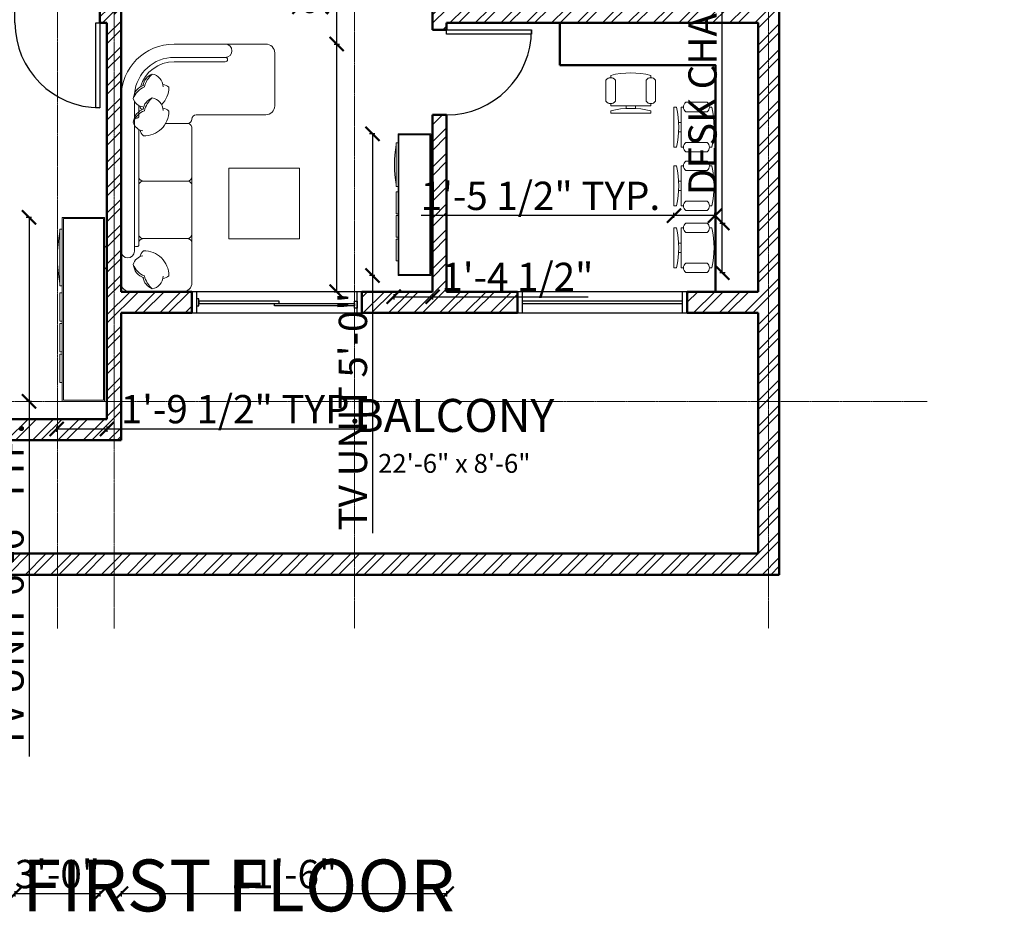
# Model space of a CAD drawing. Units: inches. Extents: x 261 to 2725, y 291 to 1454.
# Tile 23 of 35: x 1407 to 1824, y 296 to 675. Entities that reach past the tile are written whole.
import ezdxf

# ---------------------------------------------------------------- set-up
doc = ezdxf.new("R2010")
doc.units = ezdxf.units.IN
doc.linetypes.add('CENTER', pattern=[2, 1.25, -0.25, 0.25, -0.25])
for name, color, linetype, lineweight in [('A-ANNO-DIMS', 136, 'Continuous', 18), ('A-ANNO-TEXT', 7, 'Continuous', 25), ('A-AREA-IDEN', 18, 'Continuous', 18), ('A-DOOR', 160, 'Continuous', 25), ('A-FLOR-FIXT', 145, 'Continuous', 18), ('A-FURN', 30, 'Continuous', 18), ('A-GLAZ', 150, 'Continuous', 25), ('A-GRID', 251, 'CENTER', 13), ('A-WALL', 222, 'Continuous', 50), ('A-WALL-PATT', 243, 'Continuous', 13)]:
    doc.layers.add(name, color=color, linetype=linetype, lineweight=lineweight)
doc.styles.get("Standard").update_dxf_attribs({"font": 'arial.ttf'})
doc.dimstyles.new('ISO-25', dxfattribs={"dimtxt": 12, "dimasz": 6, "dimexe": 1.25, "dimexo": 0.625, "dimtad": 1, "dimdec": 0, "dimlunit": 3, "dimtxsty": 'Standard', "dimblk": 'ARCHTICK', "dimcen": 2.5, "dimadec": 0, "dimazin": 0, "dimtfac": 1, "dimtdec": 0, "dimtmove": 0, "dimatfit": 3, "dimfxl": 1, "dimfxlon": 1, "dimarcsym": 0})

# ---------------------------------------------------------------- blocks, each defined once
blk = doc.blocks.new('*U6')
for p, q in [((-36, 0), (-36, 6)), ((0, 0), (0, 6))]:
    blk.add_line(p, q)
blk.add_lwpolyline([(0, 0), (0, -36), (-1.75, -36), (-1.75, 0)], close=True)
blk.add_arc((0, 0), 36, 180, 270)
blk = doc.blocks.new('*U13')
for p, q in [((-36, 0), (-36, 6)), ((0, 0), (0, 6))]:
    blk.add_line(p, q)
blk.add_lwpolyline([(0, 0), (0, -36), (-1.75, -36), (-1.75, 0)], close=True)
blk.add_arc((0, 0), 36, 180, 270)
blk = doc.blocks.new('A$C714C64AF')
for p, q in [((3108, 2017, -5499), (1005, 2017, -5499)), ((908, 1917, -5499), (908, 1317, -5499)), ((1365, 1867, -5499), (2793, 1867, -5499)), ((3508, 1417, -5499), (3508, 839, -5499)), ((3558, 1417, -5499), (3558, 839, -5499)), ((3708, 1417, -5499), (3708, 839, -5499)), ((1008, 1217, -5499), (1458, 1217, -5499)), ((1558, 1217, -5499), (1458, 1217, -5499)), ((1558, 1217, -5499), (2760, 1217, -5499)), ((2209, 1217, -5499), (2109, 1217, -5499)), ((2908, 1167, -5499), (2908, 381, -5499)), ((3708, 839, -5499), (3708, 381, -5499)), ((3008, 281, -5499), (3608, 281, -5499))]:
    blk.add_line(p, q)
at = {"elevation": -5499}
for points in [[(940, 1667, -0.14773), (1086, 1753, -0.213343), (1215, 1879)], [(1058, 1544, 0.165541), (1089, 1478, 0.425989), (1370, 1765, 0.121523), (1303, 1804)], [(1066, 1760, -0.306663), (1215, 1879, -0.30633), (1312, 1770)], [(1456, 1817), (1438, 1817, -0.414214), (1418, 1837), (1418, 1847, -0.414214), (1438, 1867)], [(1458, 1817, -0.414214), (1508, 1767)], [(1558, 1817, 0.414214), (1508, 1767), (1508, 1267, 0.432452)], [(1558, 1817, 0.414214), (1508, 1767)], [(2670, 1867), (1884, 1867, 0.414214)], [(2109, 1817, -0.414214), (2159, 1767)], [(2209, 1817, 0.414214), (2159, 1767), (2159, 1267, 0.432452)], [(2209, 1817, 0.414214), (2159, 1767)], [(2982, 1544, -0.165541), (2951, 1478, -0.425989), (2670, 1765, -0.121523), (2737, 1804)], [(2974, 1760, 0.306663), (2825, 1879, 0.30633), (2727, 1770)], [(3068, 1867), (2753, 1867, 0.415492)], [(3100, 1667, 0.14773), (2954, 1753, 0.213343), (2825, 1879)], [(3013, 1867), (2891, 1867, 0.414214), (2871, 1847), (2871, 1837, 0.414214), (2891, 1817), (2963, 1817, 0.414214)], [(2964, 1785, -0.071865), (3006, 1804)], [(3243, 1760, 0.306663), (3094, 1879, 0.30633), (2997, 1770)], [(3369, 1667, 0.14773), (3223, 1753, 0.213343), (3094, 1879)], [(1083, 1541, -0.356772), (940, 1667, -0.249542), (1070, 1771)], [(2957, 1541, 0.356772), (3100, 1667, 0.249542), (2970, 1771)], [(3226, 1541, 0.356772), (3369, 1667, 0.249542), (3239, 1771)], [(3251, 1544, -0.165541), (3220, 1478, -0.200231), (3022, 1559)]]:
    blk.add_lwpolyline(points, format="xyb", dxfattribs=at)
for points in [[(1458, 1817), (2743, 1817)], [(1884, 1867), (2670, 1867)], [(2944, 1817), (3012, 1817)], [(2810, 1515), (2810, 1267)]]:
    blk.add_lwpolyline(points, dxfattribs=at)
blk.add_lwpolyline([(2306, 800), (1506, 800), (1506, 0), (2306, 0)], close=True, dxfattribs=at)
for centre, radius, start, end in [((1008, 1917, -5499), 100, 90, 180), ((1365, 1942, -5499), 75, 90, 270), ((3108, 1417, -5499), 600, 0, 90), ((3108, 1417, -5499), 450, 0, 84.5853), ((3108, 1417, -5499), 400, 0, 72.9371), ((1008, 1317, -5499), 100, 180, 270), ((1458, 1267, -5499), 50, 270, 0), ((1458, 1267, -5499), 50, 270, 0), ((1558, 1267, -5499), 50, 180, 270), ((1558, 1267, -5499), 50, 180, 270), ((2109, 1267, -5499), 50, 270, 0), ((2109, 1267, -5499), 50, 270, 0), ((2209, 1267, -5499), 50, 180, 270), ((2209, 1267, -5499), 50, 180, 270), ((2760, 1267, -5499), 50, 270, 0), ((2760, 1267, -5499), 50, 270, 0), ((2860, 1267, -5499), 50, 180, 270), ((2860, 1267, -5499), 50, 180, 270), ((2858, 1167, -5499), 50, 0, 90), ((3533, 839, -5499), 25, 180, 0), ((3633, 839, -5499), 75, 180, 0), ((3008, 381, -5499), 100, 180, 270), ((3608, 381, -5499), 100, 270, 0)]:
    blk.add_arc(centre, radius, start, end)
blk = doc.blocks.new('Entertainment Center')
for p, q in [((-4, 0), (-5, -1)), ((4, 0), (-4, 0)), ((5, -1), (4, 0)), ((-17, -19), (-17, -1)), ((-17, -1), (61, -1)), ((-16.5, -18.5), (-16.5, -1.5)), ((-16.5, -1.5), (60.5, -1.5)), ((60.5, -1.5), (60.5, -18.5)), ((61, -1), (61, -19)), ((61, -19), (-17, -19)), ((60.5, -18.5), (-16.5, -18.5)), ((-12, -20), (-12, -19)), ((12, -20), (-12, -20)), ((12, -19), (12, -20)), ((15, -20), (15, -19)), ((27, -20), (15, -20)), ((27, -19), (27, -20)), ((28, -20), (28, -19)), ((40, -20), (28, -20)), ((40, -19), (40, -20)), ((41, -20), (41, -19)), ((53, -20), (41, -20)), ((53, -19), (53, -20))]:
    blk.add_line(p, q)
blk.add_arc((0, 40), 61, 259.6111, 280.3889)
blk = doc.blocks.new('Chair - Desk')
for p, q in [((-8.5, 0), (-8.5, -1)), ((-8.5, 0), (8.5, 0)), ((8.5, 0), (8.5, -1)), ((-8.5, -3), (-8.5, -4)), ((-8.5, -3), (8.5, -3)), ((-2, -3), (-2, -1.9355)), ((2, -1.9576), (2, -3)), ((8.5, -3), (8.5, -4)), ((-10.5, -5), (-10.5, -14)), ((-6.5, -14), (-6.5, -5)), ((6.5, -5), (6.5, -14)), ((10.5, -14), (10.5, -5)), ((-8.5, -15), (-8.5, -16)), ((8.5, -15), (8.5, -16))]:
    blk.add_line(p, q)
for centre, radius, start, end in [((-8.5, -6.5), 2.5, 36.8699, 143.1301), ((0, 34.625), 36.625, 256.5803, 283.4197), ((8.5, -6.5), 2.5, 36.8699, 143.1301), ((-8.5, -12.5), 2.5, 216.8699, 323.1301), ((0, 19.625), 36.625, 256.5803, 283.4197), ((8.5, -12.5), 2.5, 216.8699, 323.1301)]:
    blk.add_arc(centre, radius, start, end)
blk = doc.blocks.new('WIN-72')
for p, q in [((955.45, 950.47), (946.45, 950.47)), ((950.45, 950.47), (950.45, 882.47)), ((951.45, 882.47), (951.45, 950.47)), ((946.45, 882.47), (955.45, 882.47))]:
    blk.add_line(p, q)
blk.add_lwpolyline([(955.45, 880.47), (955.45, 952.47), (946.45, 952.47), (946.45, 880.47)], close=True)
blk = doc.blocks.new('DOOR-SLIDING-72')
for p, q in [((1632.08, 973.47), (1632.08, 964.47)), ((1700.08, 964.47), (1700.08, 973.47))]:
    blk.add_line(p, q)
for points in [[(1702.08, 964.47), (1702.08, 973.47), (1630.08, 973.47), (1630.08, 964.47)], [(1632.08, 967.47), (1633.08, 967.47), (1633.08, 970.47), (1632.08, 970.47)], [(1633.08, 968.47), (1667.08, 968.47), (1667.08, 969.47), (1633.08, 969.47)], [(1699.08, 967.47), (1665.08, 967.47), (1665.08, 968.47), (1699.08, 968.47)], [(1700.08, 966.47), (1699.08, 966.47), (1699.08, 969.47), (1700.08, 969.47)]]:
    blk.add_lwpolyline(points, close=True)
blk = doc.blocks.new('_ArchTick')
at = {"color": 0, "linetype": 'ByBlock', "const_width": 0.15}
blk.add_lwpolyline([(-0.5, -0.5), (0.5, 0.5)], dxfattribs=at)
blk = doc.blocks.new('*D43')
at = {"layer": 'A-ANNO-DIMS', "color": 0, "lineweight": -2, "ltscale": 0.07, "transparency": 16777216}
for p, q in [((1412.05, 590.97), (1409.8, 590.97)), ((1411.05, 590.97), (1411.05, 512.97)), ((1412.05, 512.97), (1409.8, 512.97)), ((1411.05, 512.97), (1411.05, 362.42))]:
    blk.add_line(p, q, dxfattribs=at)
at = {"layer": 'Defpoints', "color": 0, "ltscale": 0.07, "transparency": 16777216}
for p in [(1422.75, 590.97), (1411.05, 512.97), (1422.75, 512.97)]:
    blk.add_point(p, dxfattribs=at)
at = {"layer": 'A-ANNO-DIMS', "color": 0, "lineweight": -2, "ltscale": 0.07, "transparency": 16777216, "xscale": 6, "yscale": 6, "zscale": 6}
for p, rotation in [((1411.05, 590.97), 90), ((1411.05, 512.97), 270)]:
    blk.add_blockref('_ArchTick', p, dxfattribs=dict(at, rotation=rotation))
at = {"layer": 'A-ANNO-DIMS', "color": 0, "ltscale": 0.07, "transparency": 16777216, "insert": (1404.29, 434.7), "char_height": 12, "attachment_point": 5, "rotation": 90}
blk.add_mtext('TV UNIT 6\'-6" TYP.', dxfattribs=at)
blk = doc.blocks.new('*D44')
at = {"layer": 'A-ANNO-DIMS', "color": 0, "lineweight": -2, "ltscale": 0.07, "transparency": 16777216}
for p, q in [((1422.75, 502.27), (1422.75, 500.02)), ((1422.75, 501.27), (1444.08, 501.27)), ((1444.08, 502.27), (1444.08, 500.02)), ((1444.08, 501.27), (1551.31, 501.27))]:
    blk.add_line(p, q, dxfattribs=at)
at = {"layer": 'Defpoints', "color": 0, "ltscale": 0.07, "transparency": 16777216}
for p in [(1422.75, 512.97), (1444.08, 512.97), (1444.08, 501.27)]:
    blk.add_point(p, dxfattribs=at)
at = {"layer": 'A-ANNO-DIMS', "color": 0, "lineweight": -2, "ltscale": 0.07, "transparency": 16777216, "xscale": 6, "yscale": 6, "zscale": 6, "rotation": 180}
blk.add_blockref('_ArchTick', (1422.75, 501.27), dxfattribs=at)
at = {"layer": 'A-ANNO-DIMS', "color": 0, "lineweight": -2, "ltscale": 0.07, "transparency": 16777216, "xscale": 6, "yscale": 6, "zscale": 6}
blk.add_blockref('_ArchTick', (1444.08, 501.27), dxfattribs=at)
at = {"layer": 'A-ANNO-DIMS', "color": 0, "ltscale": 0.07, "transparency": 16777216, "insert": (1500.69, 508.1), "char_height": 12, "attachment_point": 5}
blk.add_mtext('1\'-9 1/2" TYP.', dxfattribs=at)
blk = doc.blocks.new('*D45')
at = {"layer": 'A-ANNO-DIMS', "color": 0, "lineweight": -2, "ltscale": 0.07, "transparency": 16777216}
for p, q in [((1557.65, 626.41), (1555.4, 626.41)), ((1556.65, 626.41), (1556.65, 566.36)), ((1557.65, 566.36), (1555.4, 566.36)), ((1556.65, 566.36), (1556.65, 457.06))]:
    blk.add_line(p, q, dxfattribs=at)
at = {"layer": 'Defpoints', "color": 0, "ltscale": 0.07, "transparency": 16777216}
for p in [(1565.66, 626.41), (1556.65, 566.36), (1565.66, 566.36)]:
    blk.add_point(p, dxfattribs=at)
at = {"layer": 'A-ANNO-DIMS', "color": 0, "lineweight": -2, "ltscale": 0.07, "transparency": 16777216, "xscale": 6, "yscale": 6, "zscale": 6}
for p, rotation in [((1556.65, 626.41), 90), ((1556.65, 566.36), 270)]:
    blk.add_blockref('_ArchTick', p, dxfattribs=dict(at, rotation=rotation))
at = {"layer": 'A-ANNO-DIMS', "color": 0, "ltscale": 0.07, "transparency": 16777216, "insert": (1549.9, 508.71), "char_height": 12, "attachment_point": 5, "rotation": 90}
blk.add_mtext('TV UNIT 5\'-0"', dxfattribs=at)
blk = doc.blocks.new('*D46')
at = {"layer": 'A-ANNO-DIMS', "color": 0, "lineweight": -2, "ltscale": 0.07, "transparency": 16777216}
for p, q in [((1565.66, 558.35), (1565.66, 556.1)), ((1565.66, 557.35), (1582.08, 557.35)), ((1582.08, 558.35), (1582.08, 556.1)), ((1582.08, 557.35), (1648.06, 557.35))]:
    blk.add_line(p, q, dxfattribs=at)
at = {"layer": 'Defpoints', "color": 0, "ltscale": 0.07, "transparency": 16777216}
for p in [(1565.66, 566.36), (1582.08, 566.36), (1582.08, 557.35)]:
    blk.add_point(p, dxfattribs=at)
at = {"layer": 'A-ANNO-DIMS', "color": 0, "lineweight": -2, "ltscale": 0.07, "transparency": 16777216, "xscale": 6, "yscale": 6, "zscale": 6, "rotation": 180}
blk.add_blockref('_ArchTick', (1565.66, 557.35), dxfattribs=at)
at = {"layer": 'A-ANNO-DIMS', "color": 0, "lineweight": -2, "ltscale": 0.07, "transparency": 16777216, "xscale": 6, "yscale": 6, "zscale": 6}
blk.add_blockref('_ArchTick', (1582.08, 557.35), dxfattribs=at)
at = {"layer": 'A-ANNO-DIMS', "color": 0, "ltscale": 0.07, "transparency": 16777216, "insert": (1618.07, 564.18), "char_height": 12, "attachment_point": 5}
blk.add_mtext('1\'-4 1/2"', dxfattribs=at)
blk = doc.blocks.new('*D49')
at = {"layer": 'A-ANNO-DIMS', "color": 0, "lineweight": -2, "ltscale": 0.07, "transparency": 16777216}
for p, q in [((1704.93, 588.57), (1704.93, 775.49)), ((1703.93, 588.57), (1706.18, 588.57)), ((1704.93, 567.57), (1704.93, 588.57)), ((1703.93, 567.57), (1706.18, 567.57))]:
    blk.add_line(p, q, dxfattribs=at)
at = {"layer": 'Defpoints', "color": 0, "ltscale": 0.07, "transparency": 16777216}
for p in [(1701.78, 588.57), (1704.93, 588.57), (1701.78, 567.57)]:
    blk.add_point(p, dxfattribs=at)
at = {"layer": 'A-ANNO-DIMS', "color": 0, "lineweight": -2, "ltscale": 0.07, "transparency": 16777216, "xscale": 6, "yscale": 6, "zscale": 6}
for p, rotation in [((1704.93, 588.57), 90), ((1704.93, 567.57), 270)]:
    blk.add_blockref('_ArchTick', p, dxfattribs=dict(at, rotation=rotation))
at = {"layer": 'A-ANNO-DIMS', "color": 0, "ltscale": 0.07, "transparency": 16777216, "insert": (1698.1, 685.03), "char_height": 12, "attachment_point": 5, "rotation": 90}
blk.add_mtext('DESK CHAIR 1\'-9" TYP.', dxfattribs=at)
blk = doc.blocks.new('*D50')
at = {"layer": 'A-ANNO-DIMS', "color": 0, "lineweight": -2, "ltscale": 0.07, "transparency": 16777216}
for p, q in [((1684.45, 590.72), (1684.45, 592.97)), ((1701.78, 590.72), (1701.78, 592.97)), ((1684.45, 591.72), (1577.22, 591.72)), ((1701.78, 591.72), (1684.45, 591.72))]:
    blk.add_line(p, q, dxfattribs=at)
at = {"layer": 'Defpoints', "color": 0, "ltscale": 0.07, "transparency": 16777216}
for p in [(1684.45, 591.72), (1684.45, 588.57), (1701.78, 588.57)]:
    blk.add_point(p, dxfattribs=at)
at = {"layer": 'A-ANNO-DIMS', "color": 0, "lineweight": -2, "ltscale": 0.07, "transparency": 16777216, "xscale": 6, "yscale": 6, "zscale": 6, "rotation": 180}
blk.add_blockref('_ArchTick', (1684.45, 591.72), dxfattribs=at)
at = {"layer": 'A-ANNO-DIMS', "color": 0, "lineweight": -2, "ltscale": 0.07, "transparency": 16777216, "xscale": 6, "yscale": 6, "zscale": 6}
blk.add_blockref('_ArchTick', (1701.78, 591.72), dxfattribs=at)
at = {"layer": 'A-ANNO-DIMS', "color": 0, "ltscale": 0.07, "transparency": 16777216, "insert": (1627.84, 598.55), "char_height": 12, "attachment_point": 5}
blk.add_mtext('1\'-5 1/2" TYP.', dxfattribs=at)
blk = doc.blocks.new('*D55')
at = {"layer": 'A-ANNO-DIMS', "color": 0, "lineweight": -2, "ltscale": 0.07, "transparency": 16777216}
for p, q in [((1541.46, 664.47), (1541.46, 832.37)), ((1540.46, 664.47), (1542.71, 664.47)), ((1541.46, 559.47), (1541.46, 664.47)), ((1540.46, 559.47), (1542.71, 559.47))]:
    blk.add_line(p, q, dxfattribs=at)
at = {"layer": 'Defpoints', "color": 0, "ltscale": 0.07, "transparency": 16777216}
for p in [(1525.71, 664.47), (1541.46, 664.47), (1525.71, 559.47)]:
    blk.add_point(p, dxfattribs=at)
at = {"layer": 'A-ANNO-DIMS', "color": 0, "lineweight": -2, "ltscale": 0.07, "transparency": 16777216, "xscale": 6, "yscale": 6, "zscale": 6}
for p, rotation in [((1541.46, 664.47), 90), ((1541.46, 559.47), 270)]:
    blk.add_blockref('_ArchTick', p, dxfattribs=dict(at, rotation=rotation))
at = {"layer": 'A-ANNO-DIMS', "color": 0, "ltscale": 0.07, "transparency": 16777216, "insert": (1534.63, 751.42), "char_height": 12, "attachment_point": 5, "rotation": 90}
blk.add_mtext('SOFA SET 8\'-9" TYP.', dxfattribs=at)
blk = doc.blocks.new('*D56')
at = {"layer": 'A-ANNO-DIMS', "color": 0, "lineweight": -2, "ltscale": 0.07, "transparency": 16777216}
for p, q in [((1450.08, 679.22), (1450.08, 681.47)), ((1525.71, 679.22), (1525.71, 681.47)), ((1450.08, 680.22), (1341.66, 680.22)), ((1525.71, 680.22), (1450.08, 680.22))]:
    blk.add_line(p, q, dxfattribs=at)
at = {"layer": 'Defpoints', "color": 0, "ltscale": 0.07, "transparency": 16777216}
for p in [(1450.08, 680.22), (1450.08, 664.47), (1525.71, 664.47)]:
    blk.add_point(p, dxfattribs=at)
at = {"layer": 'A-ANNO-DIMS', "color": 0, "lineweight": -2, "ltscale": 0.07, "transparency": 16777216, "xscale": 6, "yscale": 6, "zscale": 6, "rotation": 180}
blk.add_blockref('_ArchTick', (1450.08, 680.22), dxfattribs=at)
at = {"layer": 'A-ANNO-DIMS', "color": 0, "lineweight": -2, "ltscale": 0.07, "transparency": 16777216, "xscale": 6, "yscale": 6, "zscale": 6}
blk.add_blockref('_ArchTick', (1525.71, 680.22), dxfattribs=at)
at = {"layer": 'A-ANNO-DIMS', "color": 0, "ltscale": 0.07, "transparency": 16777216, "insert": (1392.87, 687.05), "char_height": 12, "attachment_point": 5}
blk.add_mtext('6\'-3 1/2" TYP.', dxfattribs=at)
blk = doc.blocks.new('*D82')
at = {"layer": 'A-ANNO-DIMS', "color": 0, "lineweight": -2, "ltscale": 0.07, "transparency": 16777216}
for p, q in [((2600.96, 679.47), (2603.21, 679.47)), ((2601.96, 517.47), (2601.96, 679.47)), ((2600.96, 517.47), (2603.21, 517.47))]:
    blk.add_line(p, q, dxfattribs=at)
at = {"layer": 'Defpoints', "color": 0, "ltscale": 0.07, "transparency": 16777216}
for p in [(946.45, 679.47), (2601.96, 679.47), (946.45, 517.47)]:
    blk.add_point(p, dxfattribs=at)
at = {"layer": 'A-ANNO-DIMS', "color": 0, "lineweight": -2, "ltscale": 0.07, "transparency": 16777216, "xscale": 6, "yscale": 6, "zscale": 6}
for p, rotation in [((2601.96, 679.47), 90), ((2601.96, 517.47), 270)]:
    blk.add_blockref('_ArchTick', p, dxfattribs=dict(at, rotation=rotation))
at = {"layer": 'A-ANNO-DIMS', "color": 0, "ltscale": 0.07, "transparency": 16777216, "insert": (2595.2, 598.47), "char_height": 12, "attachment_point": 5, "rotation": 90}
blk.add_mtext('13\'-6"', dxfattribs=at)
blk = doc.blocks.new('*D89')
at = {"layer": 'A-ANNO-DIMS', "color": 0, "lineweight": -2, "ltscale": 0.07, "transparency": 16777216}
for p, q in [((2600.96, 508.47), (2603.21, 508.47)), ((2601.96, 412.47), (2601.96, 508.47)), ((2600.96, 412.47), (2603.21, 412.47))]:
    blk.add_line(p, q, dxfattribs=at)
at = {"layer": 'Defpoints', "color": 0, "ltscale": 0.07, "transparency": 16777216}
for p in [(955.45, 508.47), (2601.96, 508.47), (994.45, 412.47)]:
    blk.add_point(p, dxfattribs=at)
at = {"layer": 'A-ANNO-DIMS', "color": 0, "lineweight": -2, "ltscale": 0.07, "transparency": 16777216, "xscale": 6, "yscale": 6, "zscale": 6}
for p, rotation in [((2601.96, 508.47), 90), ((2601.96, 412.47), 270)]:
    blk.add_blockref('_ArchTick', p, dxfattribs=dict(at, rotation=rotation))
at = {"layer": 'A-ANNO-DIMS', "color": 0, "ltscale": 0.07, "transparency": 16777216, "insert": (2595.21, 460.47), "char_height": 12, "attachment_point": 5, "rotation": 90}
blk.add_mtext('8\'-0"', dxfattribs=at)
blk = doc.blocks.new('*D111')
at = {"layer": 'A-ANNO-DIMS', "color": 0, "lineweight": -2, "ltscale": 0.07, "transparency": 16777216}
for p, q in [((2600.96, 550.47), (2603.21, 550.47)), ((2601.96, 448.47), (2601.96, 550.47)), ((2600.96, 448.47), (2603.21, 448.47))]:
    blk.add_line(p, q, dxfattribs=at)
at = {"layer": 'Defpoints', "color": 0, "ltscale": 0.07, "transparency": 16777216}
for p in [(1720.08, 550.47), (2601.96, 550.47), (1720.08, 448.47)]:
    blk.add_point(p, dxfattribs=at)
at = {"layer": 'A-ANNO-DIMS', "color": 0, "lineweight": -2, "ltscale": 0.07, "transparency": 16777216, "xscale": 6, "yscale": 6, "zscale": 6}
for p, rotation in [((2601.96, 550.47), 90), ((2601.96, 448.47), 270)]:
    blk.add_blockref('_ArchTick', p, dxfattribs=dict(at, rotation=rotation))
at = {"layer": 'A-ANNO-DIMS', "color": 0, "ltscale": 0.07, "transparency": 16777216, "insert": (2595.21, 499.47), "char_height": 12, "attachment_point": 5, "rotation": 90}
blk.add_mtext('8\'-6"', dxfattribs=at)
blk = doc.blocks.new('*D112')
at = {"layer": 'A-ANNO-DIMS', "color": 0, "lineweight": -2, "ltscale": 0.07, "transparency": 16777216}
for p, q in [((2600.96, 679.47), (2603.21, 679.47)), ((2601.96, 550.47), (2601.96, 679.47)), ((2600.96, 550.47), (2603.21, 550.47))]:
    blk.add_line(p, q, dxfattribs=at)
at = {"layer": 'Defpoints', "color": 0, "ltscale": 0.07, "transparency": 16777216}
for p in [(1720.08, 679.47), (2601.96, 679.47), (1720.08, 550.47)]:
    blk.add_point(p, dxfattribs=at)
at = {"layer": 'A-ANNO-DIMS', "color": 0, "lineweight": -2, "ltscale": 0.07, "transparency": 16777216, "xscale": 6, "yscale": 6, "zscale": 6}
for p, rotation in [((2601.96, 679.47), 90), ((2601.96, 550.47), 270)]:
    blk.add_blockref('_ArchTick', p, dxfattribs=dict(at, rotation=rotation))
at = {"layer": 'A-ANNO-DIMS', "color": 0, "ltscale": 0.07, "transparency": 16777216, "insert": (2595.21, 614.97), "char_height": 12, "attachment_point": 5, "rotation": 90}
blk.add_mtext('10\'-9"', dxfattribs=at)
blk = doc.blocks.new('*D116')
at = {"layer": 'A-ANNO-DIMS', "color": 0, "lineweight": -2, "ltscale": 0.07, "transparency": 16777216}
for p, q in [((1450.08, 305.22), (1450.08, 302.97)), ((1588.08, 305.22), (1588.08, 302.97)), ((1450.08, 304.22), (1588.08, 304.22))]:
    blk.add_line(p, q, dxfattribs=at)
at = {"layer": 'Defpoints', "color": 0, "ltscale": 0.07, "transparency": 16777216}
for p in [(1588.08, 559.47), (1450.08, 550.47), (1588.08, 304.22)]:
    blk.add_point(p, dxfattribs=at)
at = {"layer": 'A-ANNO-DIMS', "color": 0, "lineweight": -2, "ltscale": 0.07, "transparency": 16777216, "xscale": 6, "yscale": 6, "zscale": 6, "rotation": 180}
blk.add_blockref('_ArchTick', (1450.08, 304.22), dxfattribs=at)
at = {"layer": 'A-ANNO-DIMS', "color": 0, "lineweight": -2, "ltscale": 0.07, "transparency": 16777216, "xscale": 6, "yscale": 6, "zscale": 6}
blk.add_blockref('_ArchTick', (1588.08, 304.22), dxfattribs=at)
at = {"layer": 'A-ANNO-DIMS', "color": 0, "ltscale": 0.07, "transparency": 16777216, "insert": (1519.08, 310.97), "char_height": 12, "attachment_point": 5}
blk.add_mtext('11\'-6"', dxfattribs=at)
blk = doc.blocks.new('*D117')
at = {"layer": 'A-ANNO-DIMS', "color": 0, "lineweight": -2, "ltscale": 0.07, "transparency": 16777216}
for p, q in [((1588.08, 1437.76), (1588.08, 1440.01)), ((1702.08, 1437.76), (1702.08, 1440.01)), ((1588.08, 1438.76), (1702.08, 1438.76))]:
    blk.add_line(p, q, dxfattribs=at)
at = {"layer": 'Defpoints', "color": 0, "ltscale": 0.07, "transparency": 16777216}
for p in [(1702.08, 1438.76), (1588.08, 559.47), (1702.08, 559.47)]:
    blk.add_point(p, dxfattribs=at)
at = {"layer": 'A-ANNO-DIMS', "color": 0, "lineweight": -2, "ltscale": 0.07, "transparency": 16777216, "xscale": 6, "yscale": 6, "zscale": 6, "rotation": 180}
blk.add_blockref('_ArchTick', (1588.08, 1438.76), dxfattribs=at)
at = {"layer": 'A-ANNO-DIMS', "color": 0, "lineweight": -2, "ltscale": 0.07, "transparency": 16777216, "xscale": 6, "yscale": 6, "zscale": 6}
blk.add_blockref('_ArchTick', (1702.08, 1438.76), dxfattribs=at)
at = {"layer": 'A-ANNO-DIMS', "color": 0, "ltscale": 0.07, "transparency": 16777216, "insert": (1645.08, 1445.51), "char_height": 12, "attachment_point": 5}
blk.add_mtext('9\'-6"', dxfattribs=at)
blk = doc.blocks.new('*D121')
at = {"layer": 'A-ANNO-DIMS', "color": 0, "lineweight": -2, "ltscale": 0.07, "transparency": 16777216}
for p, q in [((1405.08, 305.22), (1405.08, 302.97)), ((1441.08, 305.22), (1441.08, 302.97)), ((1405.08, 304.22), (1441.08, 304.22))]:
    blk.add_line(p, q, dxfattribs=at)
at = {"layer": 'Defpoints', "color": 0, "ltscale": 0.07, "transparency": 16777216}
for p in [(1405.08, 673.47), (1441.08, 673.47), (1441.08, 304.22)]:
    blk.add_point(p, dxfattribs=at)
at = {"layer": 'A-ANNO-DIMS', "color": 0, "lineweight": -2, "ltscale": 0.07, "transparency": 16777216, "xscale": 6, "yscale": 6, "zscale": 6, "rotation": 180}
blk.add_blockref('_ArchTick', (1405.08, 304.22), dxfattribs=at)
at = {"layer": 'A-ANNO-DIMS', "color": 0, "lineweight": -2, "ltscale": 0.07, "transparency": 16777216, "xscale": 6, "yscale": 6, "zscale": 6}
blk.add_blockref('_ArchTick', (1441.08, 304.22), dxfattribs=at)
at = {"layer": 'A-ANNO-DIMS', "color": 0, "ltscale": 0.07, "transparency": 16777216, "insert": (1423.08, 310.97), "char_height": 12, "attachment_point": 5}
blk.add_mtext('3\'-0"', dxfattribs=at)
blk = doc.blocks.new('*D123')
at = {"layer": 'A-ANNO-DIMS', "color": 0, "lineweight": -2, "ltscale": 0.07, "transparency": 16777216}
for p, q in [((287.06, 1054.85), (284.81, 1054.85)), ((286.06, 439.47), (286.06, 1054.85)), ((287.06, 439.47), (284.81, 439.47))]:
    blk.add_line(p, q, dxfattribs=at)
at = {"layer": 'Defpoints', "color": 0, "ltscale": 0.07, "transparency": 16777216}
for p in [(286.06, 1054.85), (2007.71, 1054.85), (2007.71, 439.47)]:
    blk.add_point(p, dxfattribs=at)
at = {"layer": 'A-ANNO-DIMS', "color": 0, "lineweight": -2, "ltscale": 0.07, "transparency": 16777216, "xscale": 6, "yscale": 6, "zscale": 6}
for p, rotation in [((286.06, 1054.85), 90), ((286.06, 439.47), 270)]:
    blk.add_blockref('_ArchTick', p, dxfattribs=dict(at, rotation=rotation))
at = {"layer": 'A-ANNO-DIMS', "color": 0, "ltscale": 0.07, "transparency": 16777216, "insert": (279.22, 747.16), "char_height": 12, "attachment_point": 5, "rotation": 90}
blk.add_mtext('51\'-3 1/2"', dxfattribs=at)

msp = doc.modelspace()

# ---------------------------------------------------------------- hatches: boundary and pattern name
at = {"layer": 'A-WALL-PATT'}
h = msp.add_hatch(dxfattribs=at)
h.set_pattern_fill('ANSI32', color=256, scale=0.8)
h.paths.add_polyline_path([(478.45, 685.47), (580.45, 685.47), (580.45, 691.47), (577.45, 691.47), (577.45, 694.47), (571.45, 694.47), (571.45, 691.47), (478.45, 691.47), (478.45, 721.47), (469.45, 721.47), (469.45, 508.47), (538.45, 508.47), (538.45, 517.47), (478.45, 517.47)])
h.paths.add_polyline_path([(694.45, 517.47), (676.45, 517.47), (676.45, 646.47), (670.45, 646.47), (670.45, 517.47), (610.45, 517.47), (610.45, 508.47), (694.45, 508.47)])
h.paths.add_polyline_path([(676.45, 784.47), (478.45, 784.47), (478.45, 844.47), (469.45, 844.47), (469.45, 745.47), (478.45, 745.47), (478.45, 775.47), (571.45, 775.47), (571.45, 724.47), (577.45, 724.47), (577.45, 775.47), (670.45, 775.47), (670.45, 691.47), (610.45, 691.47), (610.45, 685.47), (670.45, 685.47), (670.45, 682.47), (676.45, 682.47)])
h.paths.add_polyline_path([(955.45, 880.47), (946.45, 880.47), (946.45, 808.47), (778.45, 808.47), (778.45, 799.47), (946.45, 799.47), (946.45, 517.47), (898.45, 517.47), (898.45, 508.47), (955.45, 508.47)])
h.paths.add_polyline_path([(778.45, 598.47), (772.45, 598.47), (772.45, 517.47), (754.45, 517.47), (754.45, 508.47), (826.45, 508.47), (826.45, 517.47), (778.45, 517.47)])
h.paths.add_polyline_path([(955.45, 1090.47), (946.45, 1090.47), (946.45, 1030.47), (817.45, 1030.47), (817.45, 1024.47), (946.45, 1024.47), (946.45, 952.47), (955.45, 952.47)])
h.paths.add_polyline_path([(955.45, 1231.47), (730.45, 1231.47), (730.45, 1222.47), (772.45, 1222.47), (772.45, 1096.47), (766.45, 1096.47), (766.45, 1090.47), (772.45, 1090.47), (772.45, 1006.47), (712.45, 1006.47), (712.45, 1000.47), (778.45, 1000.47), (778.45, 1024.47), (781.45, 1024.47), (781.45, 1030.47), (778.45, 1030.47), (778.45, 1222.47), (946.45, 1222.47), (946.45, 1162.47), (955.45, 1162.47)])
h.paths.add_polyline_path([(694.45, 1231.47), (619.45, 1231.47), (619.45, 1222.47), (646.45, 1222.47), (646.45, 1039.47), (652.45, 1039.47), (652.45, 1090.47), (736.45, 1090.47), (736.45, 1096.47), (652.45, 1096.47), (652.45, 1222.47), (694.45, 1222.47)])
h.paths.add_polyline_path([(571.45, 1231.47), (469.45, 1231.47), (469.45, 1099.47), (478.45, 1099.47), (478.45, 1144.47), (544.45, 1144.47), (544.45, 1153.47), (538.45, 1153.47), (538.45, 1150.47), (478.45, 1150.47), (478.45, 1222.47), (538.45, 1222.47), (538.45, 1183.47), (544.45, 1183.47), (544.45, 1222.47), (571.45, 1222.47)])
h.paths.add_polyline_path([(538.45, 1006.47), (478.45, 1006.47), (478.45, 1051.47), (469.45, 1051.47), (469.45, 940.47), (478.45, 940.47), (478.45, 1000.47), (538.45, 1000.47)])
h.paths.add_polyline_path([(652.45, 1006.47), (652.45, 1009.47), (646.45, 1009.47), (646.45, 1006.47), (586.45, 1006.47), (586.45, 1000.47), (652.45, 1000.47)])
h.paths.add_polyline_path([(1288.08, 973.47), (1243.08, 973.47), (1243.08, 920.97), (1252.08, 920.97), (1252.08, 964.47), (1288.08, 964.47)], flags=17)
h.paths.add_polyline_path([(1402.08, 805.47), (1252.08, 805.47), (1252.08, 848.97), (1243.08, 848.97), (1243.08, 757.47), (1252.08, 757.47), (1252.08, 799.47), (1294.08, 799.47), (1372.08, 799.47), (1372.08, 779.47), (1372.08, 715.47), (1378.08, 715.47), (1378.08, 799.47), (1402.08, 799.47)])
h.paths.add_polyline_path([(1252.08, 721.47), (1243.08, 721.47), (1243.08, 439.47), (1729.08, 439.47), (1729.08, 709.47), (1720.08, 709.47), (1720.08, 679.47), (1582.08, 679.47), (1582.08, 670.47), (1588.08, 670.47), (1588.08, 673.47), (1720.08, 673.47), (1720.08, 559.47), (1690.08, 559.47), (1690.08, 550.47), (1720.08, 550.47), (1720.08, 448.47), (1252.08, 448.47), (1252.08, 496.47), (1312.08, 496.47), (1312.08, 505.47), (1252.08, 505.47), (1252.08, 673.47), (1405.08, 673.47), (1405.08, 679.47), (1378.08, 679.47), (1378.08, 685.47), (1372.08, 685.47), (1372.08, 679.47), (1252.08, 679.47)])
h.paths.add_polyline_path([(1450.08, 550.47), (1480.08, 550.47), (1480.08, 559.47), (1450.08, 559.47), (1450.08, 679.47), (1441.08, 679.47), (1441.08, 673.47), (1444.08, 673.47), (1444.08, 505.47), (1384.08, 505.47), (1384.08, 496.47), (1450.08, 496.47)], flags=17)
h.paths.add_polyline_path([(1618.08, 559.47), (1588.08, 559.47), (1588.08, 634.47), (1582.08, 634.47), (1582.08, 559.47), (1552.08, 559.47), (1552.08, 550.47), (1618.08, 550.47)], flags=17)
h.paths.add_polyline_path([(1564.08, 964.47), (1630.08, 964.47), (1630.08, 973.47), (1477.08, 973.47), (1477.08, 964.47), (1558.08, 964.47), (1558.08, 926.22), (1558.08, 887.97), (1486.08, 887.97), (1486.08, 881.97), (1558.08, 881.97), (1558.08, 805.47), (1450.08, 805.47), (1450.08, 845.97), (1444.08, 845.97), (1444.08, 805.47), (1438.08, 805.47), (1438.08, 799.47), (1564.08, 799.47)], flags=17)
h.paths.add_polyline_path([(1453.08, 973.47), (1408.08, 973.47), (1408.08, 964.47), (1444.08, 964.47), (1444.08, 881.97), (1450.08, 881.97), (1456.08, 881.97), (1456.08, 887.97), (1450.08, 887.97), (1450.08, 964.47), (1453.08, 964.47)], flags=17)
h.paths.add_polyline_path([(1729.08, 1231.47), (1243.08, 1231.47), (1243.08, 1167.47), (1252.08, 1167.47), (1252.08, 1222.47), (1441.08, 1222.47), (1441.08, 1045.47), (1648.08, 1045.47), (1648.08, 1051.47), (1450.08, 1051.47), (1450.08, 1074.47), (1450.08, 1222.47), (1472.08, 1222.47), (1720.08, 1222.47), (1720.08, 1051.47), (1708.08, 1051.47), (1708.08, 1045.47), (1720.08, 1045.47), (1720.08, 973.47), (1702.08, 973.47), (1702.08, 964.47), (1720.08, 964.47), (1720.08, 769.47), (1729.08, 769.47)])
h.paths.add_polyline_path([(2493.71, 1054.85), (2007.71, 1054.85), (2007.71, 439.47), (2214.67, 439.47), (2214.67, 496.47), (2493.71, 496.47)])
h.paths.add_polyline_path([(2016.71, 1045.85), (2304.71, 1045.85), (2304.71, 841.47), (2310.71, 841.47), (2310.71, 1045.85), (2484.71, 1045.85), (2484.71, 805.47), (2310.71, 805.47), (2310.71, 811.47), (2304.71, 811.47), (2304.71, 799.47), (2484.71, 799.47), (2484.71, 679.47), (2304.71, 679.47), (2304.71, 673.47), (2484.71, 673.47), (2484.71, 505.47), (2208.67, 505.47), (2208.67, 448.47), (2016.71, 448.47), (2016.71, 799.47), (2304.71, 799.47), (2304.71, 805.47), (2016.71, 805.47)], flags=16)

# ---------------------------------------------------------------- linework, layer by layer
at = {"layer": 'A-GRID', "ltscale": 0.5}
for p, q in [((1423.08, 1330.51), (1423.08, 416.51)), ((1447.08, 1330.51), (1447.08, 416.51)), ((1549.08, 1330.47), (1549.08, 416.47)), ((1724.58, 1330.47), (1724.58, 416.47)), ((1167.93, 512.97), (1791.93, 512.97))]:
    msp.add_line(p, q, dxfattribs=at)
at = {"layer": 'A-WALL'}
for p, q in [((1729.08, 709.47), (1729.08, 439.47)), ((1441.08, 673.47), (1441.08, 679.47)), ((1450.08, 559.47), (1450.08, 679.47)), ((1582.08, 670.47), (1582.08, 679.47)), ((1441.08, 673.47), (1444.08, 673.47)), ((1444.08, 505.47), (1444.08, 673.47)), ((1588.08, 670.47), (1588.08, 673.47)), ((1636.08, 655.47), (1636.08, 673.47)), ((1588.08, 670.47), (1582.08, 670.47)), ((1582.08, 559.47), (1582.08, 634.47)), ((1588.08, 634.47), (1582.08, 634.47)), ((1588.08, 559.47), (1588.08, 634.47)), ((1450.08, 559.47), (1480.08, 559.47)), ((1480.08, 559.47), (1480.08, 550.47)), ((1552.08, 559.47), (1552.08, 550.47)), ((1552.08, 559.47), (1582.08, 559.47)), ((1588.08, 559.47), (1618.08, 559.47)), ((1618.08, 559.47), (1618.08, 550.47)), ((1690.08, 559.47), (1690.08, 550.47)), ((1690.08, 559.47), (1720.08, 559.47)), ((1450.08, 496.47), (1450.08, 550.47)), ((1450.08, 550.47), (1480.08, 550.47)), ((1552.08, 550.47), (1618.08, 550.47)), ((1690.08, 550.47), (1720.08, 550.47)), ((1720.08, 550.47), (1720.08, 448.47)), ((1384.08, 505.47), (1444.08, 505.47)), ((1384.08, 496.47), (1450.08, 496.47)), ((1252.08, 448.47), (1720.08, 448.47)), ((1243.08, 439.47), (1729.08, 439.47))]:
    msp.add_line(p, q, dxfattribs=at)
for points in [[(1588.08, 673.47), (1720.08, 673.47), (1720.08, 559.47)], [(1636.08, 655.47), (1702.08, 655.47), (1702.08, 559.47)]]:
    msp.add_lwpolyline(points, dxfattribs=at)

# ---------------------------------------------------------------- block references
at = {"layer": 'A-DOOR'}
for name, p in [('*U6', (1441.08, 673.47)), ('DOOR-SLIDING-72', (-150, -414))]:
    msp.add_blockref(name, p, dxfattribs=at)
at = {"layer": 'A-DOOR', "rotation": 89.99999999999999}
msp.add_blockref('*U13', (1588.08, 670.47), dxfattribs=at)
at = {"layer": 'A-FLOR-FIXT'}
for name, p, rotation in [('Chair - Desk', (1666.11, 635.21), 180), ('Chair - Desk', (1684.45, 629.27), 90), ('Chair - Desk', (1684.45, 604.35), 90), ('Entertainment Center', (1444.08, 573.97), 270), ('Chair - Desk', (1684.45, 578.07), 90)]:
    msp.add_blockref(name, p, dxfattribs=dict(at, rotation=rotation))
at = {"layer": 'A-FLOR-FIXT', "xscale": 0.7698540399479464, "yscale": 0.7698540399479464, "zscale": 0.7698540399479464, "rotation": 270}
msp.add_blockref('Entertainment Center', (1582.08, 613.32), dxfattribs=at)
at = {"layer": 'A-FURN', "xscale": 0.0375, "yscale": 0.0375, "zscale": 0.0375, "rotation": 90.00000000000003}
msp.add_blockref('A$C714C64AF', (1525.71, 525.42, 206.2), dxfattribs=at)
at = {"layer": 'A-GLAZ', "rotation": 269.9999999999998}
msp.add_blockref('WIN-72', (737.61, 1505.92), dxfattribs=at)

# ---------------------------------------------------------------- texts
at = {"layer": 'A-ANNO-TEXT', "insert": (1369.44, 318.69), "char_height": 22, "attachment_point": 1}
msp.add_mtext_dynamic_manual_height_columns('\\pxqc;{\\fTimes New Roman|b0|i0|c0|p18;FIRST FLOOR}', width=260.751, gutter_width=12.5, heights=[0], dxfattribs=at)
at = {"layer": 'A-AREA-IDEN', "insert": (1523.88, 514), "char_height": 8, "attachment_point": 1}
msp.add_mtext_dynamic_manual_height_columns('\\pxqc;{\\fTimes New Roman|b0|i0|c0|p18;\\H1.75x;\\T1.6;BALCONY\\P\\H0.57143x;\\T1;22\'-6" x 8\'-6"}', width=134.8415, gutter_width=12.5, heights=[0], dxfattribs=at)

# ---------------------------------------------------------------- dimensions: what is measured, and where the dimension line sits
at = {"layer": 'A-ANNO-DIMS', "ltscale": 0.07}
for base, p1, p2, override, picture, middle in [((1702.08, 1438.76), (1588.08, 559.47), (1702.08, 559.47), {"dimdec": 1, "dimlfac": 1, "dimrnd": 0, "dimzin": 1, "dimdsep": 46, "dimlunit": 4, "dimfrac": 2}, '*D117', (1645.08, 1445.51)), ((1441.08, 304.22), (1405.08, 673.47), (1441.08, 673.47), {"dimdec": 1, "dimlfac": 1, "dimrnd": 0, "dimzin": 1, "dimdsep": 46, "dimlunit": 4, "dimfrac": 2}, '*D121', (1423.08, 310.97)), ((1582.08, 557.35), (1565.66, 566.36), (1582.08, 566.36), {"dimdec": 1, "dimrnd": 0, "dimzin": 1, "dimlunit": 4, "dimfrac": 2}, '*D46', (1618.07, 564.18)), ((1588.08, 304.22), (1450.08, 550.47), (1588.08, 559.47), {"dimdec": 1, "dimlfac": 1, "dimrnd": 0, "dimzin": 1, "dimdsep": 46, "dimlunit": 4, "dimfrac": 2}, '*D116', (1519.08, 310.97))]:
    dim = msp.add_linear_dim(base=base, p1=p1, p2=p2, dimstyle='ISO-25', override=override, dxfattribs=at)
    dim.commit()
    dim.dimension.update_dxf_attribs({"geometry": picture, "text_midpoint": middle})
for base, p1, p2, picture, middle in [((286.06, 1054.85), (2007.71, 439.47), (2007.71, 1054.85), '*D123', (279.22, 747.16)), ((2601.96, 679.47), (946.45, 517.47), (946.45, 679.47), '*D82', (2595.2, 598.47)), ((2601.96, 679.47), (1720.08, 550.47), (1720.08, 679.47), '*D112', (2595.21, 614.97)), ((2601.96, 550.47), (1720.08, 448.47), (1720.08, 550.47), '*D111', (2595.21, 499.47)), ((2601.96, 508.47), (994.45, 412.47), (955.45, 508.47), '*D89', (2595.21, 460.47))]:
    dim = msp.add_linear_dim(base=base, p1=p1, p2=p2, angle=90, dimstyle='ISO-25', override={"dimdec": 1, "dimlfac": 1, "dimrnd": 0, "dimzin": 1, "dimdsep": 46, "dimlunit": 4, "dimfrac": 2}, dxfattribs=at)
    dim.commit()
    dim.dimension.update_dxf_attribs({"geometry": picture, "text_midpoint": middle})
for base, p1, p2, angle, text, picture, middle in [((1541.46, 664.47), (1525.71, 559.47), (1525.71, 664.47), 90, 'SOFA SET <> TYP.', '*D55', (1534.63, 751.42)), ((1704.93, 588.57), (1701.78, 567.57), (1701.78, 588.57), 90, 'DESK CHAIR <> TYP.', '*D49', (1698.1, 685.03)), ((1450.08, 680.22), (1525.71, 664.47), (1450.08, 664.47), 180, '<> TYP.', '*D56', (1392.87, 687.05)), ((1556.6487, 566.3619), (1565.656, 626.4105), (1565.656, 566.3619), 270, 'TV UNIT <>', '*D45', (1549.8968, 508.7123)), ((1684.45, 591.72), (1701.78, 588.57), (1684.45, 588.57), 180, '<> TYP.', '*D50', (1627.84, 598.55)), ((1411.05, 512.97), (1422.75, 590.97), (1422.75, 512.97), 270, 'TV UNIT <> TYP.', '*D43', (1404.29, 434.7))]:
    dim = msp.add_linear_dim(base=base, p1=p1, p2=p2, angle=angle, text=text, dimstyle='ISO-25', override={"dimdec": 1, "dimrnd": 0, "dimzin": 1, "dimlunit": 4, "dimfrac": 2}, dxfattribs=at)
    dim.commit()
    dim.dimension.update_dxf_attribs({"geometry": picture, "text_midpoint": middle})
dim = msp.add_linear_dim(base=(1444.08, 501.27), p1=(1422.75, 512.97), p2=(1444.08, 512.97), text='<> TYP.', dimstyle='ISO-25', override={"dimdec": 1, "dimrnd": 0, "dimzin": 1, "dimlunit": 4, "dimfrac": 2}, dxfattribs=at)
dim.commit()
dim.dimension.update_dxf_attribs({"geometry": '*D44', "text_midpoint": (1500.69, 508.1)})

doc.saveas('drawing.dxf')
